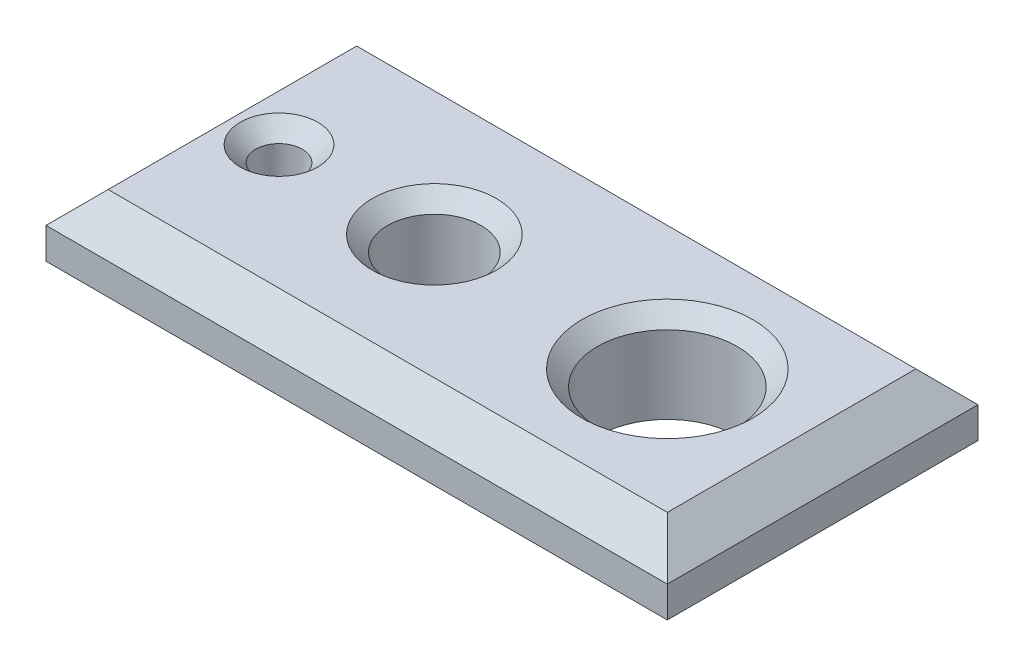
ISO-10303-21;
HEADER;
FILE_DESCRIPTION(('STEP AP214'),'2;1');
FILE_NAME('part.step','',(''),(''),'','','');
FILE_SCHEMA(('AUTOMOTIVE_DESIGN { 1 0 10303 214 1 1 1 1 }'));
ENDSEC;
DATA;
#1=APPLICATION_CONTEXT('core data for automotive mechanical design processes');
#2=APPLICATION_PROTOCOL_DEFINITION('international standard','automotive_design',2000,#1);
#3=PRODUCT_CONTEXT('',#1,'mechanical');
#4=PRODUCT('Part','Part','',(#3));
#5=PRODUCT_RELATED_PRODUCT_CATEGORY('part','',(#4));
#6=PRODUCT_DEFINITION_FORMATION('','',#4);
#7=PRODUCT_DEFINITION_CONTEXT('part definition',#1,'design');
#8=PRODUCT_DEFINITION('design','',#6,#7);
#9=PRODUCT_DEFINITION_SHAPE('','',#8);
#10=(LENGTH_UNIT() NAMED_UNIT(*) SI_UNIT(.MILLI.,.METRE.));
#11=(NAMED_UNIT(*) PLANE_ANGLE_UNIT() SI_UNIT($,.RADIAN.));
#12=(NAMED_UNIT(*) SI_UNIT($,.STERADIAN.) SOLID_ANGLE_UNIT());
#13=UNCERTAINTY_MEASURE_WITH_UNIT(LENGTH_MEASURE(1.E-05),#10,'distance_accuracy_value','');
#14=(GEOMETRIC_REPRESENTATION_CONTEXT(3) GLOBAL_UNCERTAINTY_ASSIGNED_CONTEXT((#13)) GLOBAL_UNIT_ASSIGNED_CONTEXT((#10,
#11,#12)) REPRESENTATION_CONTEXT('',''));
#15=CARTESIAN_POINT('',(0.,0.,0.));
#16=DIRECTION('',(0.,0.,1.));
#17=DIRECTION('',(1.,0.,0.));
#18=AXIS2_PLACEMENT_3D('',#15,#16,#17);
#19=CARTESIAN_POINT('',(100.,15.,50.));
#20=DIRECTION('',(-1.,0.,0.));
#21=DIRECTION('',(0.,0.,1.));
#22=AXIS2_PLACEMENT_3D('',#19,#20,#21);
#23=PLANE('',#22);
#24=DIRECTION('',(0.,-1.,0.));
#25=VECTOR('',#24,1.);
#26=CARTESIAN_POINT('',(100.,15.,50.));
#27=LINE('',#26,#25);
#28=CARTESIAN_POINT('',(100.,4.99999999999994,50.));
#29=VERTEX_POINT('',#28);
#30=CARTESIAN_POINT('',(100.,-4.99999999999996,50.));
#31=VERTEX_POINT('',#30);
#32=EDGE_CURVE('E278',#29,#31,#27,.T.);
#33=ORIENTED_EDGE('',*,*,#32,.T.);
#34=DIRECTION('',(0.,0.,-1.));
#35=VECTOR('',#34,1.);
#36=CARTESIAN_POINT('',(100.,-4.99999999999996,-50.));
#37=LINE('',#36,#35);
#38=CARTESIAN_POINT('',(100.,-4.99999999999996,-50.));
#39=VERTEX_POINT('',#38);
#40=EDGE_CURVE('E270',#31,#39,#37,.T.);
#41=ORIENTED_EDGE('',*,*,#40,.T.);
#42=DIRECTION('',(0.,-1.,0.));
#43=VECTOR('',#42,1.);
#44=CARTESIAN_POINT('',(100.,15.,-50.));
#45=LINE('',#44,#43);
#46=CARTESIAN_POINT('',(100.,4.99999999999994,-50.));
#47=VERTEX_POINT('',#46);
#48=EDGE_CURVE('E133',#47,#39,#45,.T.);
#49=ORIENTED_EDGE('',*,*,#48,.F.);
#50=DIRECTION('',(0.,0.,1.));
#51=VECTOR('',#50,1.);
#52=CARTESIAN_POINT('',(100.,4.99999999999994,50.));
#53=LINE('',#52,#51);
#54=EDGE_CURVE('E305',#47,#29,#53,.T.);
#55=ORIENTED_EDGE('',*,*,#54,.T.);
#56=EDGE_LOOP('',(#33,#41,#49,#55));
#57=FACE_BOUND('',#56,.T.);
#58=ADVANCED_FACE('F41',(#57),#23,.F.);
#59=CARTESIAN_POINT('',(-100.,15.,-50.));
#60=DIRECTION('',(0.,0.,1.));
#61=DIRECTION('',(1.,0.,0.));
#62=AXIS2_PLACEMENT_3D('',#59,#60,#61);
#63=PLANE('',#62);
#64=ORIENTED_EDGE('',*,*,#48,.T.);
#65=DIRECTION('',(-1.,0.,0.));
#66=VECTOR('',#65,1.);
#67=CARTESIAN_POINT('',(-100.,-4.99999999999996,-50.));
#68=LINE('',#67,#66);
#69=CARTESIAN_POINT('',(-100.,-4.99999999999996,-50.));
#70=VERTEX_POINT('',#69);
#71=EDGE_CURVE('E128',#39,#70,#68,.T.);
#72=ORIENTED_EDGE('',*,*,#71,.T.);
#73=DIRECTION('',(0.,-1.,0.));
#74=VECTOR('',#73,1.);
#75=CARTESIAN_POINT('',(-100.,15.,-50.));
#76=LINE('',#75,#74);
#77=CARTESIAN_POINT('',(-100.,4.99999999999994,-50.));
#78=VERTEX_POINT('',#77);
#79=EDGE_CURVE('E112',#78,#70,#76,.T.);
#80=ORIENTED_EDGE('',*,*,#79,.F.);
#81=DIRECTION('',(1.,0.,0.));
#82=VECTOR('',#81,1.);
#83=CARTESIAN_POINT('',(-100.,4.99999999999994,-50.));
#84=LINE('',#83,#82);
#85=EDGE_CURVE('E130',#78,#47,#84,.T.);
#86=ORIENTED_EDGE('',*,*,#85,.T.);
#87=EDGE_LOOP('',(#64,#72,#80,#86));
#88=FACE_BOUND('',#87,.T.);
#89=ADVANCED_FACE('F127',(#88),#63,.F.);
#90=CARTESIAN_POINT('',(-100.,15.,50.));
#91=DIRECTION('',(1.,0.,0.));
#92=DIRECTION('',(0.,0.,-1.));
#93=AXIS2_PLACEMENT_3D('',#90,#91,#92);
#94=PLANE('',#93);
#95=ORIENTED_EDGE('',*,*,#79,.T.);
#96=DIRECTION('',(0.,0.,1.));
#97=VECTOR('',#96,1.);
#98=CARTESIAN_POINT('',(-100.,-4.99999999999996,50.));
#99=LINE('',#98,#97);
#100=CARTESIAN_POINT('',(-100.,-4.99999999999996,50.));
#101=VERTEX_POINT('',#100);
#102=EDGE_CURVE('E116',#70,#101,#99,.T.);
#103=ORIENTED_EDGE('',*,*,#102,.T.);
#104=DIRECTION('',(0.,-1.,0.));
#105=VECTOR('',#104,1.);
#106=CARTESIAN_POINT('',(-100.,15.,50.));
#107=LINE('',#106,#105);
#108=CARTESIAN_POINT('',(-100.,4.99999999999994,50.));
#109=VERTEX_POINT('',#108);
#110=EDGE_CURVE('E114',#109,#101,#107,.T.);
#111=ORIENTED_EDGE('',*,*,#110,.F.);
#112=DIRECTION('',(0.,0.,-1.));
#113=VECTOR('',#112,1.);
#114=CARTESIAN_POINT('',(-100.,4.99999999999994,50.));
#115=LINE('',#114,#113);
#116=EDGE_CURVE('E107',#109,#78,#115,.T.);
#117=ORIENTED_EDGE('',*,*,#116,.T.);
#118=EDGE_LOOP('',(#95,#103,#111,#117));
#119=FACE_BOUND('',#118,.T.);
#120=ADVANCED_FACE('F109',(#119),#94,.F.);
#121=CARTESIAN_POINT('',(-100.,15.,50.));
#122=DIRECTION('',(0.,0.,-1.));
#123=DIRECTION('',(-1.,0.,0.));
#124=AXIS2_PLACEMENT_3D('',#121,#122,#123);
#125=PLANE('',#124);
#126=ORIENTED_EDGE('',*,*,#110,.T.);
#127=DIRECTION('',(1.,0.,0.));
#128=VECTOR('',#127,1.);
#129=CARTESIAN_POINT('',(100.,-4.99999999999996,50.));
#130=LINE('',#129,#128);
#131=EDGE_CURVE('E304',#101,#31,#130,.T.);
#132=ORIENTED_EDGE('',*,*,#131,.T.);
#133=ORIENTED_EDGE('',*,*,#32,.F.);
#134=DIRECTION('',(-1.,0.,0.));
#135=VECTOR('',#134,1.);
#136=CARTESIAN_POINT('',(-100.,4.99999999999994,50.));
#137=LINE('',#136,#135);
#138=EDGE_CURVE('E262',#29,#109,#137,.T.);
#139=ORIENTED_EDGE('',*,*,#138,.T.);
#140=EDGE_LOOP('',(#126,#132,#133,#139));
#141=FACE_BOUND('',#140,.T.);
#142=ADVANCED_FACE('F313',(#141),#125,.F.);
#143=CARTESIAN_POINT('',(0.,15.,0.));
#144=DIRECTION('',(0.,-1.,0.));
#145=DIRECTION('',(0.,0.,-1.));
#146=AXIS2_PLACEMENT_3D('',#143,#144,#145);
#147=PLANE('',#146);
#148=CARTESIAN_POINT('',(50.,15.,0.));
#149=DIRECTION('',(0.,-1.,0.));
#150=DIRECTION('',(0.,0.,-1.));
#151=AXIS2_PLACEMENT_3D('',#148,#149,#150);
#152=CIRCLE('',#151,27.5);
#153=CARTESIAN_POINT('',(50.,15.,-27.5));
#154=VERTEX_POINT('',#153);
#155=EDGE_CURVE('E166',#154,#154,#152,.T.);
#156=ORIENTED_EDGE('',*,*,#155,.T.);
#157=EDGE_LOOP('',(#156));
#158=FACE_BOUND('',#157,.T.);
#159=CARTESIAN_POINT('',(-25.,15.,0.));
#160=DIRECTION('',(0.,-1.,0.));
#161=DIRECTION('',(0.,0.,-1.));
#162=AXIS2_PLACEMENT_3D('',#159,#160,#161);
#163=CIRCLE('',#162,20.);
#164=CARTESIAN_POINT('',(-25.,15.,-20.));
#165=VERTEX_POINT('',#164);
#166=EDGE_CURVE('E167',#165,#165,#163,.T.);
#167=ORIENTED_EDGE('',*,*,#166,.T.);
#168=EDGE_LOOP('',(#167));
#169=FACE_BOUND('',#168,.T.);
#170=CARTESIAN_POINT('',(-75.,15.,0.));
#171=DIRECTION('',(0.,-1.,0.));
#172=DIRECTION('',(0.,0.,-1.));
#173=AXIS2_PLACEMENT_3D('',#170,#171,#172);
#174=CIRCLE('',#173,12.5);
#175=CARTESIAN_POINT('',(-75.,15.,-12.5));
#176=VERTEX_POINT('',#175);
#177=EDGE_CURVE('E165',#176,#176,#174,.T.);
#178=ORIENTED_EDGE('',*,*,#177,.T.);
#179=EDGE_LOOP('',(#178));
#180=FACE_BOUND('',#179,.T.);
#181=DIRECTION('',(0.,0.,-1.));
#182=VECTOR('',#181,1.);
#183=CARTESIAN_POINT('',(90.,15.,0.));
#184=LINE('',#183,#182);
#185=CARTESIAN_POINT('',(90.,15.,40.));
#186=VERTEX_POINT('',#185);
#187=CARTESIAN_POINT('',(90.,15.,-40.));
#188=VERTEX_POINT('',#187);
#189=EDGE_CURVE('E60',#186,#188,#184,.T.);
#190=ORIENTED_EDGE('',*,*,#189,.T.);
#191=DIRECTION('',(-1.,0.,0.));
#192=VECTOR('',#191,1.);
#193=CARTESIAN_POINT('',(0.,15.,-40.));
#194=LINE('',#193,#192);
#195=CARTESIAN_POINT('',(-90.,15.,-40.));
#196=VERTEX_POINT('',#195);
#197=EDGE_CURVE('E162',#188,#196,#194,.T.);
#198=ORIENTED_EDGE('',*,*,#197,.T.);
#199=DIRECTION('',(0.,0.,1.));
#200=VECTOR('',#199,1.);
#201=CARTESIAN_POINT('',(-90.,15.,0.));
#202=LINE('',#201,#200);
#203=CARTESIAN_POINT('',(-90.,15.,40.));
#204=VERTEX_POINT('',#203);
#205=EDGE_CURVE('E142',#196,#204,#202,.T.);
#206=ORIENTED_EDGE('',*,*,#205,.T.);
#207=DIRECTION('',(1.,0.,0.));
#208=VECTOR('',#207,1.);
#209=CARTESIAN_POINT('',(0.,15.,40.));
#210=LINE('',#209,#208);
#211=EDGE_CURVE('E65',#204,#186,#210,.T.);
#212=ORIENTED_EDGE('',*,*,#211,.T.);
#213=EDGE_LOOP('',(#190,#198,#206,#212));
#214=FACE_BOUND('',#213,.T.);
#215=ADVANCED_FACE('F312',(#158,#169,#180,#214),#147,.F.);
#216=CARTESIAN_POINT('',(0.,-15.,0.));
#217=DIRECTION('',(0.,-1.,0.));
#218=DIRECTION('',(0.,0.,-1.));
#219=AXIS2_PLACEMENT_3D('',#216,#217,#218);
#220=PLANE('',#219);
#221=CARTESIAN_POINT('',(-75.,-15.,0.));
#222=DIRECTION('',(0.,-1.,0.));
#223=DIRECTION('',(0.,0.,-1.));
#224=AXIS2_PLACEMENT_3D('',#221,#222,#223);
#225=CIRCLE('',#224,7.50000000000001);
#226=CARTESIAN_POINT('',(-75.,-15.,-7.50000000000001));
#227=VERTEX_POINT('',#226);
#228=EDGE_CURVE('E141',#227,#227,#225,.F.);
#229=ORIENTED_EDGE('',*,*,#228,.T.);
#230=EDGE_LOOP('',(#229));
#231=FACE_BOUND('',#230,.T.);
#232=CARTESIAN_POINT('',(-25.,-15.,0.));
#233=DIRECTION('',(0.,-1.,0.));
#234=DIRECTION('',(0.,0.,-1.));
#235=AXIS2_PLACEMENT_3D('',#232,#233,#234);
#236=CIRCLE('',#235,15.);
#237=CARTESIAN_POINT('',(-25.,-15.,-15.));
#238=VERTEX_POINT('',#237);
#239=EDGE_CURVE('E146',#238,#238,#236,.F.);
#240=ORIENTED_EDGE('',*,*,#239,.T.);
#241=EDGE_LOOP('',(#240));
#242=FACE_BOUND('',#241,.T.);
#243=CARTESIAN_POINT('',(50.,-15.,0.));
#244=DIRECTION('',(0.,-1.,0.));
#245=DIRECTION('',(0.,0.,-1.));
#246=AXIS2_PLACEMENT_3D('',#243,#244,#245);
#247=CIRCLE('',#246,22.5);
#248=CARTESIAN_POINT('',(50.,-15.,-22.5));
#249=VERTEX_POINT('',#248);
#250=EDGE_CURVE('E289',#249,#249,#247,.F.);
#251=ORIENTED_EDGE('',*,*,#250,.T.);
#252=EDGE_LOOP('',(#251));
#253=FACE_BOUND('',#252,.T.);
#254=DIRECTION('',(0.,0.,-1.));
#255=VECTOR('',#254,1.);
#256=CARTESIAN_POINT('',(-89.9999999999999,-15.,-50.));
#257=LINE('',#256,#255);
#258=CARTESIAN_POINT('',(-89.9999999999999,-15.,39.9999999999999));
#259=VERTEX_POINT('',#258);
#260=CARTESIAN_POINT('',(-89.9999999999999,-15.,-39.9999999999999));
#261=VERTEX_POINT('',#260);
#262=EDGE_CURVE('E300',#259,#261,#257,.T.);
#263=ORIENTED_EDGE('',*,*,#262,.T.);
#264=DIRECTION('',(1.,0.,0.));
#265=VECTOR('',#264,1.);
#266=CARTESIAN_POINT('',(100.,-15.,-39.9999999999999));
#267=LINE('',#266,#265);
#268=CARTESIAN_POINT('',(89.9999999999999,-15.,-39.9999999999999));
#269=VERTEX_POINT('',#268);
#270=EDGE_CURVE('E119',#261,#269,#267,.T.);
#271=ORIENTED_EDGE('',*,*,#270,.T.);
#272=DIRECTION('',(0.,0.,1.));
#273=VECTOR('',#272,1.);
#274=CARTESIAN_POINT('',(89.9999999999999,-15.,50.));
#275=LINE('',#274,#273);
#276=CARTESIAN_POINT('',(89.9999999999999,-15.,39.9999999999999));
#277=VERTEX_POINT('',#276);
#278=EDGE_CURVE('E291',#269,#277,#275,.T.);
#279=ORIENTED_EDGE('',*,*,#278,.T.);
#280=DIRECTION('',(-1.,0.,0.));
#281=VECTOR('',#280,1.);
#282=CARTESIAN_POINT('',(-100.,-15.,39.9999999999999));
#283=LINE('',#282,#281);
#284=EDGE_CURVE('E293',#277,#259,#283,.T.);
#285=ORIENTED_EDGE('',*,*,#284,.T.);
#286=EDGE_LOOP('',(#263,#271,#279,#285));
#287=FACE_BOUND('',#286,.T.);
#288=ADVANCED_FACE('F227',(#231,#242,#253,#287),#220,.T.);
#289=CARTESIAN_POINT('',(-100.,-4.99999999999996,50.));
#290=DIRECTION('',(0.,-0.707106781186548,0.707106781186546));
#291=DIRECTION('',(-1.,0.,0.));
#292=AXIS2_PLACEMENT_3D('',#289,#290,#291);
#293=PLANE('',#292);
#294=DIRECTION('',(0.577350269189626,-0.577350269189625,-0.577350269189626));
#295=VECTOR('',#294,1.);
#296=CARTESIAN_POINT('',(-100.,-4.99999999999996,50.));
#297=LINE('',#296,#295);
#298=EDGE_CURVE('E273',#259,#101,#297,.F.);
#299=ORIENTED_EDGE('',*,*,#298,.F.);
#300=ORIENTED_EDGE('',*,*,#284,.F.);
#301=DIRECTION('',(-0.577350269189626,-0.577350269189625,-0.577350269189626));
#302=VECTOR('',#301,1.);
#303=CARTESIAN_POINT('',(100.,-4.99999999999996,50.));
#304=LINE('',#303,#302);
#305=EDGE_CURVE('E151',#31,#277,#304,.T.);
#306=ORIENTED_EDGE('',*,*,#305,.F.);
#307=ORIENTED_EDGE('',*,*,#131,.F.);
#308=EDGE_LOOP('',(#299,#300,#306,#307));
#309=FACE_BOUND('',#308,.T.);
#310=ADVANCED_FACE('F221',(#309),#293,.T.);
#311=CARTESIAN_POINT('',(100.,-4.99999999999996,50.));
#312=DIRECTION('',(0.707106781186546,-0.707106781186548,0.));
#313=DIRECTION('',(0.,0.,1.));
#314=AXIS2_PLACEMENT_3D('',#311,#312,#313);
#315=PLANE('',#314);
#316=ORIENTED_EDGE('',*,*,#305,.T.);
#317=ORIENTED_EDGE('',*,*,#278,.F.);
#318=DIRECTION('',(0.577350269189626,0.577350269189625,-0.577350269189626));
#319=VECTOR('',#318,1.);
#320=CARTESIAN_POINT('',(66.6666666666666,-38.3333333333333,-16.6666666666666));
#321=LINE('',#320,#319);
#322=EDGE_CURVE('E272',#39,#269,#321,.F.);
#323=ORIENTED_EDGE('',*,*,#322,.F.);
#324=ORIENTED_EDGE('',*,*,#40,.F.);
#325=EDGE_LOOP('',(#316,#317,#323,#324));
#326=FACE_BOUND('',#325,.T.);
#327=ADVANCED_FACE('F220',(#326),#315,.T.);
#328=CARTESIAN_POINT('',(-100.,-4.99999999999996,50.));
#329=DIRECTION('',(-0.707106781186546,-0.707106781186548,0.));
#330=DIRECTION('',(0.,0.,-1.));
#331=AXIS2_PLACEMENT_3D('',#328,#329,#330);
#332=PLANE('',#331);
#333=ORIENTED_EDGE('',*,*,#298,.T.);
#334=ORIENTED_EDGE('',*,*,#102,.F.);
#335=DIRECTION('',(0.577350269189626,-0.577350269189625,0.577350269189626));
#336=VECTOR('',#335,1.);
#337=CARTESIAN_POINT('',(-66.6666666666666,-38.3333333333333,-16.6666666666666));
#338=LINE('',#337,#336);
#339=EDGE_CURVE('E158',#261,#70,#338,.F.);
#340=ORIENTED_EDGE('',*,*,#339,.F.);
#341=ORIENTED_EDGE('',*,*,#262,.F.);
#342=EDGE_LOOP('',(#333,#334,#340,#341));
#343=FACE_BOUND('',#342,.T.);
#344=ADVANCED_FACE('F209',(#343),#332,.T.);
#345=CARTESIAN_POINT('',(-100.,-4.99999999999996,-50.));
#346=DIRECTION('',(0.,-0.707106781186548,-0.707106781186546));
#347=DIRECTION('',(1.,0.,0.));
#348=AXIS2_PLACEMENT_3D('',#345,#346,#347);
#349=PLANE('',#348);
#350=ORIENTED_EDGE('',*,*,#322,.T.);
#351=ORIENTED_EDGE('',*,*,#270,.F.);
#352=ORIENTED_EDGE('',*,*,#339,.T.);
#353=ORIENTED_EDGE('',*,*,#71,.F.);
#354=EDGE_LOOP('',(#350,#351,#352,#353));
#355=FACE_BOUND('',#354,.T.);
#356=ADVANCED_FACE('F205',(#355),#349,.T.);
#357=CARTESIAN_POINT('',(0.,15.,40.));
#358=DIRECTION('',(0.,-0.707106781186545,-0.707106781186549));
#359=DIRECTION('',(1.,0.,0.));
#360=AXIS2_PLACEMENT_3D('',#357,#358,#359);
#361=PLANE('',#360);
#362=DIRECTION('',(0.577350269189625,0.577350269189628,-0.577350269189625));
#363=VECTOR('',#362,1.);
#364=CARTESIAN_POINT('',(-76.6666666666667,28.3333333333334,26.6666666666667));
#365=LINE('',#364,#363);
#366=EDGE_CURVE('E144',#109,#204,#365,.T.);
#367=ORIENTED_EDGE('',*,*,#366,.F.);
#368=ORIENTED_EDGE('',*,*,#138,.F.);
#369=DIRECTION('',(-0.577350269189625,0.577350269189628,-0.577350269189625));
#370=VECTOR('',#369,1.);
#371=CARTESIAN_POINT('',(60.0000000000001,45.0000000000001,10.0000000000001));
#372=LINE('',#371,#370);
#373=EDGE_CURVE('E154',#186,#29,#372,.F.);
#374=ORIENTED_EDGE('',*,*,#373,.F.);
#375=ORIENTED_EDGE('',*,*,#211,.F.);
#376=EDGE_LOOP('',(#367,#368,#374,#375));
#377=FACE_BOUND('',#376,.T.);
#378=ADVANCED_FACE('F207',(#377),#361,.F.);
#379=CARTESIAN_POINT('',(90.,15.,0.));
#380=DIRECTION('',(-0.707106781186549,-0.707106781186545,0.));
#381=DIRECTION('',(0.,0.,-1.));
#382=AXIS2_PLACEMENT_3D('',#379,#380,#381);
#383=PLANE('',#382);
#384=ORIENTED_EDGE('',*,*,#373,.T.);
#385=ORIENTED_EDGE('',*,*,#54,.F.);
#386=DIRECTION('',(-0.577350269189625,0.577350269189628,0.577350269189625));
#387=VECTOR('',#386,1.);
#388=CARTESIAN_POINT('',(76.6666666666667,28.3333333333334,-26.6666666666667));
#389=LINE('',#388,#387);
#390=EDGE_CURVE('E139',#188,#47,#389,.F.);
#391=ORIENTED_EDGE('',*,*,#390,.F.);
#392=ORIENTED_EDGE('',*,*,#189,.F.);
#393=EDGE_LOOP('',(#384,#385,#391,#392));
#394=FACE_BOUND('',#393,.T.);
#395=ADVANCED_FACE('F242',(#394),#383,.F.);
#396=CARTESIAN_POINT('',(-90.,15.,0.));
#397=DIRECTION('',(0.707106781186549,-0.707106781186545,0.));
#398=DIRECTION('',(0.,0.,1.));
#399=AXIS2_PLACEMENT_3D('',#396,#397,#398);
#400=PLANE('',#399);
#401=ORIENTED_EDGE('',*,*,#366,.T.);
#402=ORIENTED_EDGE('',*,*,#205,.F.);
#403=DIRECTION('',(-0.577350269189625,-0.577350269189628,-0.577350269189625));
#404=VECTOR('',#403,1.);
#405=CARTESIAN_POINT('',(-76.6666666666667,28.3333333333334,-26.6666666666667));
#406=LINE('',#405,#404);
#407=EDGE_CURVE('E136',#78,#196,#406,.F.);
#408=ORIENTED_EDGE('',*,*,#407,.F.);
#409=ORIENTED_EDGE('',*,*,#116,.F.);
#410=EDGE_LOOP('',(#401,#402,#408,#409));
#411=FACE_BOUND('',#410,.T.);
#412=ADVANCED_FACE('F143',(#411),#400,.F.);
#413=CARTESIAN_POINT('',(0.,15.,-40.));
#414=DIRECTION('',(0.,-0.707106781186545,0.707106781186549));
#415=DIRECTION('',(-1.,0.,0.));
#416=AXIS2_PLACEMENT_3D('',#413,#414,#415);
#417=PLANE('',#416);
#418=ORIENTED_EDGE('',*,*,#390,.T.);
#419=ORIENTED_EDGE('',*,*,#85,.F.);
#420=ORIENTED_EDGE('',*,*,#407,.T.);
#421=ORIENTED_EDGE('',*,*,#197,.F.);
#422=EDGE_LOOP('',(#418,#419,#420,#421));
#423=FACE_BOUND('',#422,.T.);
#424=ADVANCED_FACE('F134',(#423),#417,.F.);
#425=CARTESIAN_POINT('',(50.,-78.6396103067893,0.));
#426=DIRECTION('',(0.,1.,0.));
#427=DIRECTION('',(0.,0.,1.));
#428=AXIS2_PLACEMENT_3D('',#425,#426,#427);
#429=CYLINDRICAL_SURFACE('',#428,22.5);
#430=CARTESIAN_POINT('',(50.,9.99999999999999,0.));
#431=DIRECTION('',(0.,-1.,0.));
#432=DIRECTION('',(0.,0.,-1.));
#433=AXIS2_PLACEMENT_3D('',#430,#431,#432);
#434=CIRCLE('',#433,22.5);
#435=CARTESIAN_POINT('',(50.,9.99999999999999,-22.5));
#436=VERTEX_POINT('',#435);
#437=EDGE_CURVE('E157',#436,#436,#434,.F.);
#438=ORIENTED_EDGE('',*,*,#437,.T.);
#439=EDGE_LOOP('',(#438));
#440=FACE_BOUND('',#439,.T.);
#441=ORIENTED_EDGE('',*,*,#250,.F.);
#442=EDGE_LOOP('',(#441));
#443=FACE_BOUND('',#442,.T.);
#444=ADVANCED_FACE('F239',(#440,#443),#429,.F.);
#445=CARTESIAN_POINT('',(-25.,-78.6396103067893,0.));
#446=DIRECTION('',(0.,1.,0.));
#447=DIRECTION('',(0.,0.,1.));
#448=AXIS2_PLACEMENT_3D('',#445,#446,#447);
#449=CYLINDRICAL_SURFACE('',#448,15.);
#450=CARTESIAN_POINT('',(-25.,9.99999999999998,0.));
#451=DIRECTION('',(0.,-1.,0.));
#452=DIRECTION('',(0.,0.,-1.));
#453=AXIS2_PLACEMENT_3D('',#450,#451,#452);
#454=CIRCLE('',#453,15.);
#455=CARTESIAN_POINT('',(-25.,9.99999999999998,-15.));
#456=VERTEX_POINT('',#455);
#457=EDGE_CURVE('E49',#456,#456,#454,.F.);
#458=ORIENTED_EDGE('',*,*,#457,.T.);
#459=EDGE_LOOP('',(#458));
#460=FACE_BOUND('',#459,.T.);
#461=ORIENTED_EDGE('',*,*,#239,.F.);
#462=EDGE_LOOP('',(#461));
#463=FACE_BOUND('',#462,.T.);
#464=ADVANCED_FACE('F174',(#460,#463),#449,.F.);
#465=CARTESIAN_POINT('',(-75.,-78.6396103067893,0.));
#466=DIRECTION('',(0.,1.,0.));
#467=DIRECTION('',(0.,0.,1.));
#468=AXIS2_PLACEMENT_3D('',#465,#466,#467);
#469=CYLINDRICAL_SURFACE('',#468,7.50000000000001);
#470=CARTESIAN_POINT('',(-75.,10.,0.));
#471=DIRECTION('',(0.,-1.,0.));
#472=DIRECTION('',(0.,0.,-1.));
#473=AXIS2_PLACEMENT_3D('',#470,#471,#472);
#474=CIRCLE('',#473,7.50000000000001);
#475=CARTESIAN_POINT('',(-75.,10.,-7.50000000000001));
#476=VERTEX_POINT('',#475);
#477=EDGE_CURVE('E11',#476,#476,#474,.F.);
#478=ORIENTED_EDGE('',*,*,#477,.T.);
#479=EDGE_LOOP('',(#478));
#480=FACE_BOUND('',#479,.T.);
#481=ORIENTED_EDGE('',*,*,#228,.F.);
#482=EDGE_LOOP('',(#481));
#483=FACE_BOUND('',#482,.T.);
#484=ADVANCED_FACE('F188',(#480,#483),#469,.F.);
#485=CARTESIAN_POINT('',(50.,9.99999999999999,0.));
#486=DIRECTION('',(0.,1.,0.));
#487=DIRECTION('',(0.,0.,1.));
#488=AXIS2_PLACEMENT_3D('',#485,#486,#487);
#489=CONICAL_SURFACE('',#488,22.5,0.785398163397451);
#490=ORIENTED_EDGE('',*,*,#155,.F.);
#491=EDGE_LOOP('',(#490));
#492=FACE_BOUND('',#491,.T.);
#493=ORIENTED_EDGE('',*,*,#437,.F.);
#494=EDGE_LOOP('',(#493));
#495=FACE_BOUND('',#494,.T.);
#496=ADVANCED_FACE('F178',(#492,#495),#489,.F.);
#497=CARTESIAN_POINT('',(-25.,9.99999999999998,0.));
#498=DIRECTION('',(0.,1.,0.));
#499=DIRECTION('',(0.,0.,1.));
#500=AXIS2_PLACEMENT_3D('',#497,#498,#499);
#501=CONICAL_SURFACE('',#500,15.,0.785398163397448);
#502=ORIENTED_EDGE('',*,*,#166,.F.);
#503=EDGE_LOOP('',(#502));
#504=FACE_BOUND('',#503,.T.);
#505=ORIENTED_EDGE('',*,*,#457,.F.);
#506=EDGE_LOOP('',(#505));
#507=FACE_BOUND('',#506,.T.);
#508=ADVANCED_FACE('F177',(#504,#507),#501,.F.);
#509=CARTESIAN_POINT('',(-75.,10.,0.));
#510=DIRECTION('',(0.,1.,0.));
#511=DIRECTION('',(0.,0.,1.));
#512=AXIS2_PLACEMENT_3D('',#509,#510,#511);
#513=CONICAL_SURFACE('',#512,7.50000000000001,0.785398163397449);
#514=ORIENTED_EDGE('',*,*,#177,.F.);
#515=EDGE_LOOP('',(#514));
#516=FACE_BOUND('',#515,.T.);
#517=ORIENTED_EDGE('',*,*,#477,.F.);
#518=EDGE_LOOP('',(#517));
#519=FACE_BOUND('',#518,.T.);
#520=ADVANCED_FACE('F42',(#516,#519),#513,.F.);
#521=CLOSED_SHELL('',(#58,#89,#120,#142,#215,#288,#310,#327,#344,#356,#378,#395,#412,#424,#444,
#464,#484,#496,#508,#520));
#522=MANIFOLD_SOLID_BREP('B2',#521);
#523=ADVANCED_BREP_SHAPE_REPRESENTATION('',(#18,#522),#14);
#524=SHAPE_DEFINITION_REPRESENTATION(#9,#523);
ENDSEC;
END-ISO-10303-21;
